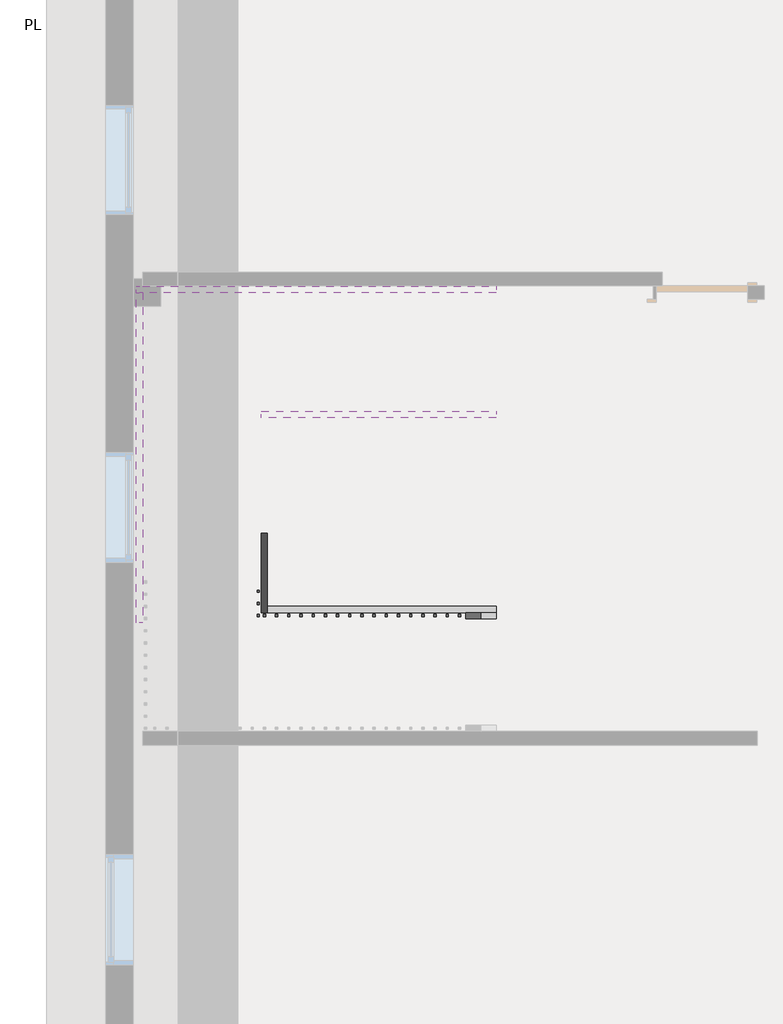
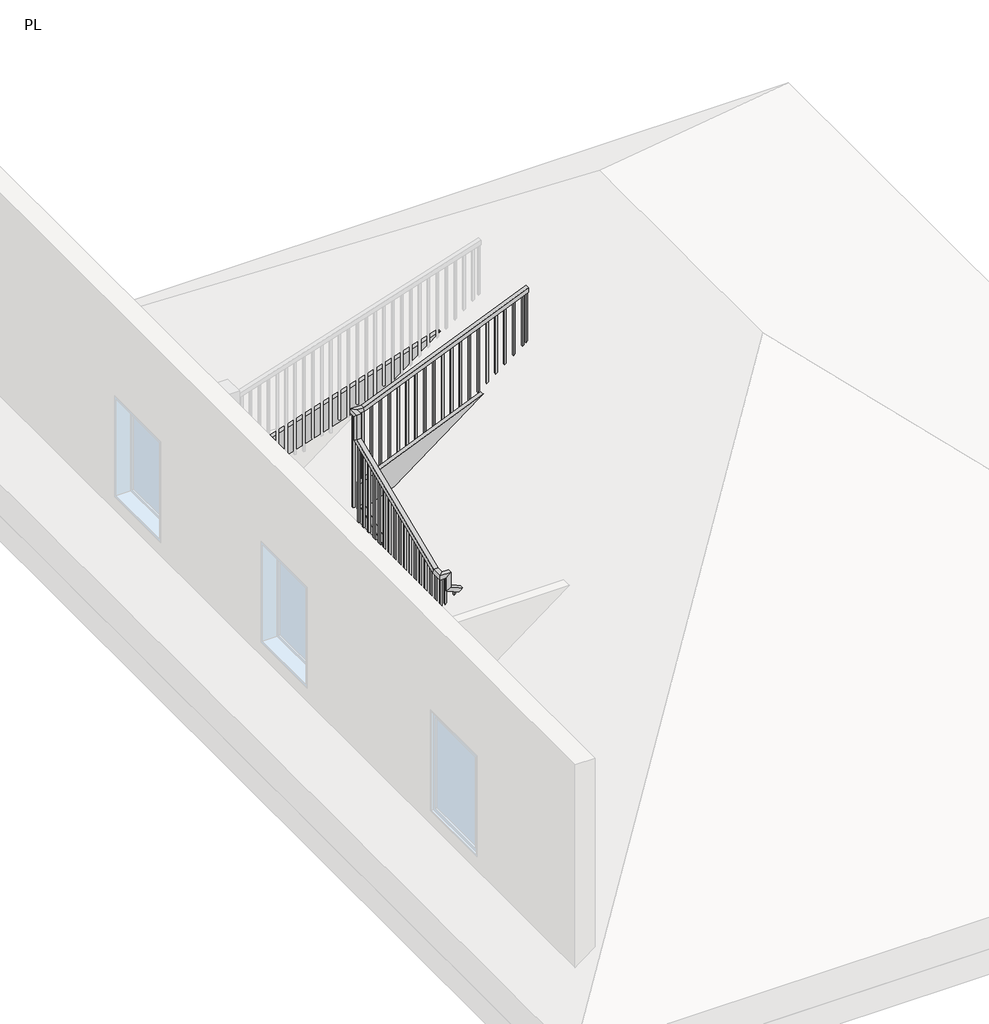
# One storey, part 3 of 3: 6 members, 1 railing.
"""IFC4 building model written with IfcOpenShell, lengths in millimetres."""

from ifc_helpers import new_model, si_unit, frame, origin, place, context, project, spatial, polyline, outline, extrude, faceted_brep, element, save

model = new_model("IFC4")

# Units and contexts
model_context = context("Model", 3, world=origin())
ifc_project = project(units=[si_unit("LENGTHUNIT", "METRE", prefix="MILLI")], contexts=[model_context])

# Site, building, storey
site = spatial("IfcSite", under=ifc_project)
building = spatial("IfcBuilding", under=site)
storey = spatial("IfcBuildingStorey", under=building, Name="PL", Elevation=0.0)

# Members
placement = place(None, origin())
element("IfcMember", 1, ObjectType="Stringer - 2\" Width", at=placement, inside=storey, context=model_context, shape_type="SweptSolid", body=[
    extrude(outline(polyline([(0.0, 5202.3334712), (314.7886477, 5202.3334712), (942.1719103, 3707.0700288), (942.1719103, 2919.2768366), (0.0, 5164.7865561), (0.0, 5202.3334712)])), frame((0.0, 4060.0450307, 0.0), z_axis=(0.0, 1.0, 0.0), x_axis=(0.0, 0.0, 1.0)), (0.0, 0.0, 1.0), 50.8),
])
element("IfcMember", 2, ObjectType="Stringer - 2\" Width", at=placement, inside=storey, context=model_context, shape_type="SweptSolid", body=[
    extrude(outline(polyline([(5015.4041654, 1220.4977979), (7768.4450307, 2067.5872949), (7768.4450307, 1748.6851248), (6051.8362182, 1220.4977979), (5015.4041654, 1220.4977979)])), frame((2205.1334712, 0.0, 0.0), z_axis=(1.0, 0.0, 0.0), x_axis=(0.0, 1.0, 0.0)), (0.0, 0.0, 1.0), 50.8),
])
element("IfcMember", 3, ObjectType="Stringer - 2\" Width", at=placement, inside=storey, context=model_context, shape_type="SweptSolid", body=[
    extrude(outline(polyline([(2051.8454089, 2205.1334712), (1748.6851248, 2205.1334712), (1748.6851248, 2257.6240611), (2685.9931599, 5202.3334712), (3005.8613241, 5202.3334712), (2051.8454089, 2205.1334712)])), frame((0.0, 7768.4450307, 0.0), z_axis=(0.0, 1.0, 0.0), x_axis=(0.0, 0.0, 1.0)), (0.0, 0.0, 1.0), 50.8),
])
element("IfcMember", 4, ObjectType="Stringer - 2\" Width", at=placement, inside=storey, context=model_context, shape_type="SweptSolid", body=[
    extrude(outline(polyline([(0.0, 5202.3334712), (314.7886477, 5202.3334712), (1114.089347, 3297.3334712), (783.5467489, 3297.3334712), (0.0, 5164.7865562), (0.0, 5202.3334712)])), frame((0.0, 5101.4450307, 0.0), z_axis=(0.0, 1.0, 0.0), x_axis=(0.0, 0.0, 1.0)), (0.0, 0.0, 1.0), 50.8),
])
element("IfcMember", 5, ObjectType="Stringer - 2\" Width", at=placement, inside=storey, context=model_context, shape_type="SweptSolid", body=[
    extrude(outline(polyline([(5101.4450307, 922.0922035), (5101.4450307, 1252.6348016), (6727.0450307, 1934.7047317), (6727.0450307, 1604.1621336), (5101.4450307, 922.0922035)])), frame((3246.5334712, 0.0, 0.0), z_axis=(1.0, 0.0, 0.0), x_axis=(0.0, 1.0, 0.0)), (0.0, 0.0, 1.0), 50.8),
])
element("IfcMember", 6, ObjectType="Stringer - 2\" Width", at=placement, inside=storey, context=model_context, shape_type="SweptSolid", body=[
    extrude(outline(polyline([(2190.4809554, 3246.5334712), (1859.9383573, 3246.5334712), (2680.5537419, 5202.3334712), (3011.0963401, 5202.3334712), (2190.4809554, 3246.5334712)])), frame((0.0, 6727.0450307, 0.0), z_axis=(0.0, 1.0, 0.0), x_axis=(0.0, 0.0, 1.0)), (0.0, 0.0, 1.0), 50.8),
])

# Railing
element("IfcRailing", 7, ObjectType="Handrail - Rectangular", at=placement, inside=storey, context=model_context, shape_type="SolidModel", body=[
    faceted_brep([(5202.3334712, 5050.6450307, 1148.8615385), (5202.3334712, 5050.6450307, 1093.7711054), (5202.3334712, 5101.4450307, 1093.7711054), (5202.3334712, 5101.4450307, 1148.8615385), (3322.7334712, 5050.6450307, 1937.5048951), (3271.9334712, 5050.6450307, 1903.7291474), (3271.9334712, 5101.4450307, 1903.7291474), (3322.7334712, 5101.4450307, 1937.5048951), (3322.7334712, 5050.6450307, 2118.6797203), (3271.9334712, 5050.6450307, 2067.8797203), (3271.9334712, 5101.4450307, 2067.8797203), (3322.7334712, 5101.4450307, 2118.6797203), (3195.7334712, 5050.6450307, 2118.6797203), (3195.7334712, 5050.6450307, 2067.8797203), (3246.5334712, 5101.4450307, 2067.8797203), (3246.5334712, 5101.4450307, 2118.6797203), (3195.7334712, 5177.6450307, 2118.6797203), (3195.7334712, 5187.8705627, 2067.8797203), (3246.5334712, 5187.8705627, 2067.8797203), (3246.5334712, 5177.6450307, 2118.6797203), (3195.7334712, 6701.6450307, 2758.1202797), (3195.7334712, 6752.4450307, 2724.344532), (3246.5334712, 6752.4450307, 2724.344532), (3246.5334712, 6701.6450307, 2758.1202797), (5202.3334712, 6828.6450307, 3845.1692308), (5202.3334712, 6777.8450307, 3845.1692308), (5202.3334712, 6777.8450307, 3790.0787978), (5202.3334712, 6828.6450307, 3790.0787978), (3332.9590032, 6828.6450307, 3005.7258741), (3322.7334712, 6828.6450307, 3056.5258741), (3332.9590032, 6777.8450307, 3005.7258741), (3322.7334712, 6777.8450307, 3056.5258741), (3195.7334712, 6701.6450307, 3056.5258741), (3195.7334712, 6752.4450307, 3005.7258741), (3246.5334712, 6752.4450307, 3005.7258741), (3246.5334712, 6701.6450307, 3056.5258741), (3195.7334712, 6828.6450307, 3056.5258741), (3195.7334712, 6828.6450307, 3005.7258741), (3246.5334712, 6777.8450307, 3005.7258741), (3246.5334712, 6777.8450307, 3056.5258741)], [[[0, 1, 2, 3]], [[1, 0, 4, 5]], [[2, 1, 5, 6]], [[3, 2, 6, 7]], [[0, 3, 7, 4]], [[5, 4, 8, 9]], [[6, 5, 9, 10]], [[7, 6, 10, 11]], [[4, 7, 11, 8]], [[9, 8, 12, 13]], [[10, 9, 13, 14]], [[11, 10, 14, 15]], [[8, 11, 15, 12]], [[13, 12, 16, 17]], [[14, 13, 17, 18]], [[15, 14, 18, 19]], [[12, 15, 19, 16]], [[17, 16, 20, 21]], [[18, 17, 21, 22]], [[19, 18, 22, 23]], [[16, 19, 23, 20]], [[24, 25, 26, 27]], [[28, 29, 24, 27]], [[30, 28, 27, 26]], [[31, 30, 26, 25]], [[29, 31, 25, 24]], [[21, 20, 32, 33]], [[22, 21, 33, 34]], [[23, 22, 34, 35]], [[20, 23, 35, 32]], [[33, 32, 36, 37]], [[34, 33, 37, 38]], [[35, 34, 38, 39]], [[32, 35, 39, 36]], [[37, 36, 29, 28]], [[38, 37, 28, 30]], [[39, 38, 30, 31]], [[36, 39, 31, 29]]]),
    extrude(outline(polyline([(3772.7606159, 5161.0584712), (3764.7676089, 5142.0084712), (2813.5384615, 5142.0084712), (2813.5384615, 5161.0584712), (3772.7606159, 5161.0584712)])), frame((0.0, 6793.7200307, 0.0), z_axis=(0.0, 1.0, 0.0), x_axis=(0.0, 0.0, 1.0)), (0.0, 0.0, 1.0), 19.05),
    extrude(outline(polyline([(3730.1312453, 5059.4584712), (3722.1382383, 5040.4084712), (2813.5384615, 5040.4084712), (2813.5384615, 5059.4584712), (3730.1312453, 5059.4584712)])), frame((0.0, 6793.7200307, 0.0), z_axis=(0.0, 1.0, 0.0), x_axis=(0.0, 0.0, 1.0)), (0.0, 0.0, 1.0), 19.05),
    extrude(outline(polyline([(3687.5018747, 4957.8584712), (3679.5088677, 4938.8084712), (2813.5384615, 4938.8084712), (2813.5384615, 4957.8584712), (3687.5018747, 4957.8584712)])), frame((0.0, 6793.7200307, 0.0), z_axis=(0.0, 1.0, 0.0), x_axis=(0.0, 0.0, 1.0)), (0.0, 0.0, 1.0), 19.05),
    extrude(outline(polyline([(3644.872504, 4856.2584712), (3636.8794971, 4837.2084712), (2696.3076923, 4837.2084712), (2696.3076923, 4856.2584712), (3644.872504, 4856.2584712)])), frame((0.0, 6793.7200307, 0.0), z_axis=(0.0, 1.0, 0.0), x_axis=(0.0, 0.0, 1.0)), (0.0, 0.0, 1.0), 19.05),
    extrude(outline(polyline([(3602.2431334, 4754.6584712), (3594.2501264, 4735.6084712), (2696.3076923, 4735.6084712), (2696.3076923, 4754.6584712), (3602.2431334, 4754.6584712)])), frame((0.0, 6793.7200307, 0.0), z_axis=(0.0, 1.0, 0.0), x_axis=(0.0, 0.0, 1.0)), (0.0, 0.0, 1.0), 19.05),
    extrude(outline(polyline([(3559.6137628, 4653.0584712), (3551.6207558, 4634.0084712), (2696.3076923, 4634.0084712), (2696.3076923, 4653.0584712), (3559.6137628, 4653.0584712)])), frame((0.0, 6793.7200307, 0.0), z_axis=(0.0, 1.0, 0.0), x_axis=(0.0, 0.0, 1.0)), (0.0, 0.0, 1.0), 19.05),
    extrude(outline(polyline([(3516.9843922, 4551.4584712), (3508.9913852, 4532.4084712), (2579.0769231, 4532.4084712), (2579.0769231, 4551.4584712), (3516.9843922, 4551.4584712)])), frame((0.0, 6793.7200307, 0.0), z_axis=(0.0, 1.0, 0.0), x_axis=(0.0, 0.0, 1.0)), (0.0, 0.0, 1.0), 19.05),
    extrude(outline(polyline([(3474.3550215, 4449.8584712), (3466.3620145, 4430.8084712), (2579.0769231, 4430.8084712), (2579.0769231, 4449.8584712), (3474.3550215, 4449.8584712)])), frame((0.0, 6793.7200307, 0.0), z_axis=(0.0, 1.0, 0.0), x_axis=(0.0, 0.0, 1.0)), (0.0, 0.0, 1.0), 19.05),
    extrude(outline(polyline([(3431.7256509, 4348.2584712), (3423.7326439, 4329.2084712), (2461.8461538, 4329.2084712), (2461.8461538, 4348.2584712), (3431.7256509, 4348.2584712)])), frame((0.0, 6793.7200307, 0.0), z_axis=(0.0, 1.0, 0.0), x_axis=(0.0, 0.0, 1.0)), (0.0, 0.0, 1.0), 19.05),
    extrude(outline(polyline([(3389.0962803, 4246.6584712), (3381.1032733, 4227.6084712), (2461.8461538, 4227.6084712), (2461.8461538, 4246.6584712), (3389.0962803, 4246.6584712)])), frame((0.0, 6793.7200307, 0.0), z_axis=(0.0, 1.0, 0.0), x_axis=(0.0, 0.0, 1.0)), (0.0, 0.0, 1.0), 19.05),
    extrude(outline(polyline([(3346.4669096, 4145.0584712), (3338.4739026, 4126.0084712), (2461.8461538, 4126.0084712), (2461.8461538, 4145.0584712), (3346.4669096, 4145.0584712)])), frame((0.0, 6793.7200307, 0.0), z_axis=(0.0, 1.0, 0.0), x_axis=(0.0, 0.0, 1.0)), (0.0, 0.0, 1.0), 19.05),
    extrude(outline(polyline([(3303.837539, 4043.4584712), (3295.844532, 4024.4084712), (2344.6153846, 4024.4084712), (2344.6153846, 4043.4584712), (3303.837539, 4043.4584712)])), frame((0.0, 6793.7200307, 0.0), z_axis=(0.0, 1.0, 0.0), x_axis=(0.0, 0.0, 1.0)), (0.0, 0.0, 1.0), 19.05),
    extrude(outline(polyline([(3261.2081684, 3941.8584712), (3253.2151614, 3922.8084712), (2344.6153846, 3922.8084712), (2344.6153846, 3941.8584712), (3261.2081684, 3941.8584712)])), frame((0.0, 6793.7200307, 0.0), z_axis=(0.0, 1.0, 0.0), x_axis=(0.0, 0.0, 1.0)), (0.0, 0.0, 1.0), 19.05),
    extrude(outline(polyline([(3218.5787978, 3840.2584712), (3210.5857908, 3821.2084712), (2344.6153846, 3821.2084712), (2344.6153846, 3840.2584712), (3218.5787978, 3840.2584712)])), frame((0.0, 6793.7200307, 0.0), z_axis=(0.0, 1.0, 0.0), x_axis=(0.0, 0.0, 1.0)), (0.0, 0.0, 1.0), 19.05),
    extrude(outline(polyline([(3175.9494271, 3738.6584712), (3167.9564201, 3719.6084712), (2227.3846154, 3719.6084712), (2227.3846154, 3738.6584712), (3175.9494271, 3738.6584712)])), frame((0.0, 6793.7200307, 0.0), z_axis=(0.0, 1.0, 0.0), x_axis=(0.0, 0.0, 1.0)), (0.0, 0.0, 1.0), 19.05),
    extrude(outline(polyline([(3133.3200565, 3637.0584712), (3125.3270495, 3618.0084712), (2227.3846154, 3618.0084712), (2227.3846154, 3637.0584712), (3133.3200565, 3637.0584712)])), frame((0.0, 6793.7200307, 0.0), z_axis=(0.0, 1.0, 0.0), x_axis=(0.0, 0.0, 1.0)), (0.0, 0.0, 1.0), 19.05),
    extrude(outline(polyline([(3090.6906859, 3535.4584712), (3082.6976789, 3516.4084712), (2227.3846154, 3516.4084712), (2227.3846154, 3535.4584712), (3090.6906859, 3535.4584712)])), frame((0.0, 6793.7200307, 0.0), z_axis=(0.0, 1.0, 0.0), x_axis=(0.0, 0.0, 1.0)), (0.0, 0.0, 1.0), 19.05),
    extrude(outline(polyline([(3048.0613152, 3433.8584712), (3040.0683082, 3414.8084712), (2110.1538462, 3414.8084712), (2110.1538462, 3433.8584712), (3048.0613152, 3433.8584712)])), frame((0.0, 6793.7200307, 0.0), z_axis=(0.0, 1.0, 0.0), x_axis=(0.0, 0.0, 1.0)), (0.0, 0.0, 1.0), 19.05),
    extrude(outline(polyline([(3005.4319446, 3332.2584712), (2997.4389376, 3313.2084712), (2110.1538462, 3313.2084712), (2110.1538462, 3332.2584712), (3005.4319446, 3332.2584712)])), frame((0.0, 6793.7200307, 0.0), z_axis=(0.0, 1.0, 0.0), x_axis=(0.0, 0.0, 1.0)), (0.0, 0.0, 1.0), 19.05),
    extrude(outline(polyline([(6692.1200307, 2699.0333432), (6711.1700307, 2707.0263502), (6711.1700307, 1758.4615385), (6692.1200307, 1758.4615385), (6692.1200307, 2699.0333432)])), frame((3211.6084712, 0.0, 0.0), z_axis=(1.0, 0.0, 0.0), x_axis=(0.0, 1.0, 0.0)), (0.0, 0.0, 1.0), 19.05),
    extrude(outline(polyline([(6590.5200307, 2656.4039726), (6609.5700307, 2664.3969796), (6609.5700307, 1758.4615385), (6590.5200307, 1758.4615385), (6590.5200307, 2656.4039726)])), frame((3211.6084712, 0.0, 0.0), z_axis=(1.0, 0.0, 0.0), x_axis=(0.0, 1.0, 0.0)), (0.0, 0.0, 1.0), 19.05),
    extrude(outline(polyline([(6488.9200307, 2613.7746019), (6507.9700307, 2621.7676089), (6507.9700307, 1758.4615385), (6488.9200307, 1758.4615385), (6488.9200307, 2613.7746019)])), frame((3211.6084712, 0.0, 0.0), z_axis=(1.0, 0.0, 0.0), x_axis=(0.0, 1.0, 0.0)), (0.0, 0.0, 1.0), 19.05),
    extrude(outline(polyline([(6387.3200307, 2571.1452313), (6406.3700307, 2579.1382383), (6406.3700307, 1641.2307692), (6387.3200307, 1641.2307692), (6387.3200307, 2571.1452313)])), frame((3211.6084712, 0.0, 0.0), z_axis=(1.0, 0.0, 0.0), x_axis=(0.0, 1.0, 0.0)), (0.0, 0.0, 1.0), 19.05),
    extrude(outline(polyline([(6285.7200307, 2528.5158607), (6304.7700307, 2536.5088677), (6304.7700307, 1641.2307692), (6285.7200307, 1641.2307692), (6285.7200307, 2528.5158607)])), frame((3211.6084712, 0.0, 0.0), z_axis=(1.0, 0.0, 0.0), x_axis=(0.0, 1.0, 0.0)), (0.0, 0.0, 1.0), 19.05),
    extrude(outline(polyline([(6184.1200307, 2485.8864901), (6203.1700307, 2493.8794971), (6203.1700307, 1524.0), (6184.1200307, 1524.0), (6184.1200307, 2485.8864901)])), frame((3211.6084712, 0.0, 0.0), z_axis=(1.0, 0.0, 0.0), x_axis=(0.0, 1.0, 0.0)), (0.0, 0.0, 1.0), 19.05),
    extrude(outline(polyline([(6082.5200307, 2443.2571194), (6101.5700307, 2451.2501264), (6101.5700307, 1524.0), (6082.5200307, 1524.0), (6082.5200307, 2443.2571194)])), frame((3211.6084712, 0.0, 0.0), z_axis=(1.0, 0.0, 0.0), x_axis=(0.0, 1.0, 0.0)), (0.0, 0.0, 1.0), 19.05),
    extrude(outline(polyline([(5980.9200307, 2400.6277488), (5999.9700307, 2408.6207558), (5999.9700307, 1524.0), (5980.9200307, 1524.0), (5980.9200307, 2400.6277488)])), frame((3211.6084712, 0.0, 0.0), z_axis=(1.0, 0.0, 0.0), x_axis=(0.0, 1.0, 0.0)), (0.0, 0.0, 1.0), 19.05),
    extrude(outline(polyline([(5879.3200307, 2357.9983782), (5898.3700307, 2365.9913852), (5898.3700307, 1406.7692308), (5879.3200307, 1406.7692308), (5879.3200307, 2357.9983782)])), frame((3211.6084712, 0.0, 0.0), z_axis=(1.0, 0.0, 0.0), x_axis=(0.0, 1.0, 0.0)), (0.0, 0.0, 1.0), 19.05),
    extrude(outline(polyline([(5777.7200307, 2315.3690075), (5796.7700307, 2323.3620145), (5796.7700307, 1406.7692308), (5777.7200307, 1406.7692308), (5777.7200307, 2315.3690075)])), frame((3211.6084712, 0.0, 0.0), z_axis=(1.0, 0.0, 0.0), x_axis=(0.0, 1.0, 0.0)), (0.0, 0.0, 1.0), 19.05),
    extrude(outline(polyline([(5676.1200307, 2272.7396369), (5695.1700307, 2280.7326439), (5695.1700307, 1406.7692308), (5676.1200307, 1406.7692308), (5676.1200307, 2272.7396369)])), frame((3211.6084712, 0.0, 0.0), z_axis=(1.0, 0.0, 0.0), x_axis=(0.0, 1.0, 0.0)), (0.0, 0.0, 1.0), 19.05),
    extrude(outline(polyline([(5574.5200307, 2230.1102663), (5593.5700307, 2238.1032733), (5593.5700307, 1289.5384615), (5574.5200307, 1289.5384615), (5574.5200307, 2230.1102663)])), frame((3211.6084712, 0.0, 0.0), z_axis=(1.0, 0.0, 0.0), x_axis=(0.0, 1.0, 0.0)), (0.0, 0.0, 1.0), 19.05),
    extrude(outline(polyline([(5472.9200307, 2187.4808957), (5491.9700307, 2195.4739026), (5491.9700307, 1289.5384615), (5472.9200307, 1289.5384615), (5472.9200307, 2187.4808957)])), frame((3211.6084712, 0.0, 0.0), z_axis=(1.0, 0.0, 0.0), x_axis=(0.0, 1.0, 0.0)), (0.0, 0.0, 1.0), 19.05),
    extrude(outline(polyline([(5371.3200307, 2144.851525), (5390.3700307, 2152.844532), (5390.3700307, 1289.5384615), (5371.3200307, 1289.5384615), (5371.3200307, 2144.851525)])), frame((3211.6084712, 0.0, 0.0), z_axis=(1.0, 0.0, 0.0), x_axis=(0.0, 1.0, 0.0)), (0.0, 0.0, 1.0), 19.05),
    extrude(outline(polyline([(5269.7200307, 2102.2221544), (5288.7700307, 2110.2151614), (5288.7700307, 1172.3076923), (5269.7200307, 1172.3076923), (5269.7200307, 2102.2221544)])), frame((3211.6084712, 0.0, 0.0), z_axis=(1.0, 0.0, 0.0), x_axis=(0.0, 1.0, 0.0)), (0.0, 0.0, 1.0), 19.05),
    extrude(outline(polyline([(5168.1200307, 2059.5927838), (5187.1700307, 2067.5857908), (5187.1700307, 1172.3076923), (5168.1200307, 1172.3076923), (5168.1200307, 2059.5927838)])), frame((3211.6084712, 0.0, 0.0), z_axis=(1.0, 0.0, 0.0), x_axis=(0.0, 1.0, 0.0)), (0.0, 0.0, 1.0), 19.05),
    extrude(outline(polyline([(3281.4584712, 5085.5700307), (3281.4584712, 5066.5200307), (3262.4084712, 5066.5200307), (3262.4084712, 5085.5700307), (3281.4584712, 5085.5700307)])), frame((0.0, 0.0, 937.8461538), z_axis=(0.0, 0.0, 1.0), x_axis=(1.0, 0.0, 0.0)), (0.0, 0.0, 1.0), 1130.0335664),
    extrude(outline(polyline([(1857.1032733, 3383.0584712), (1865.0962803, 3364.0084712), (937.8461538, 3364.0084712), (937.8461538, 3383.0584712), (1857.1032733, 3383.0584712)])), frame((0.0, 5066.5200307, 0.0), z_axis=(0.0, 1.0, 0.0), x_axis=(0.0, 0.0, 1.0)), (0.0, 0.0, 1.0), 19.05),
    extrude(outline(polyline([(1814.4739026, 3484.6584712), (1822.4669096, 3465.6084712), (937.8461538, 3465.6084712), (937.8461538, 3484.6584712), (1814.4739026, 3484.6584712)])), frame((0.0, 5066.5200307, 0.0), z_axis=(0.0, 1.0, 0.0), x_axis=(0.0, 0.0, 1.0)), (0.0, 0.0, 1.0), 19.05),
    extrude(outline(polyline([(1771.844532, 3586.2584712), (1779.837539, 3567.2084712), (820.6153846, 3567.2084712), (820.6153846, 3586.2584712), (1771.844532, 3586.2584712)])), frame((0.0, 5066.5200307, 0.0), z_axis=(0.0, 1.0, 0.0), x_axis=(0.0, 0.0, 1.0)), (0.0, 0.0, 1.0), 19.05),
    extrude(outline(polyline([(1729.2151614, 3687.8584712), (1737.2081684, 3668.8084712), (820.6153846, 3668.8084712), (820.6153846, 3687.8584712), (1729.2151614, 3687.8584712)])), frame((0.0, 5066.5200307, 0.0), z_axis=(0.0, 1.0, 0.0), x_axis=(0.0, 0.0, 1.0)), (0.0, 0.0, 1.0), 19.05),
    extrude(outline(polyline([(1686.5857908, 3789.4584712), (1694.5787978, 3770.4084712), (820.6153846, 3770.4084712), (820.6153846, 3789.4584712), (1686.5857908, 3789.4584712)])), frame((0.0, 5066.5200307, 0.0), z_axis=(0.0, 1.0, 0.0), x_axis=(0.0, 0.0, 1.0)), (0.0, 0.0, 1.0), 19.05),
    extrude(outline(polyline([(1643.9564201, 3891.0584712), (1651.9494271, 3872.0084712), (703.3846154, 3872.0084712), (703.3846154, 3891.0584712), (1643.9564201, 3891.0584712)])), frame((0.0, 5066.5200307, 0.0), z_axis=(0.0, 1.0, 0.0), x_axis=(0.0, 0.0, 1.0)), (0.0, 0.0, 1.0), 19.05),
    extrude(outline(polyline([(1601.3270495, 3992.6584712), (1609.3200565, 3973.6084712), (703.3846154, 3973.6084712), (703.3846154, 3992.6584712), (1601.3270495, 3992.6584712)])), frame((0.0, 5066.5200307, 0.0), z_axis=(0.0, 1.0, 0.0), x_axis=(0.0, 0.0, 1.0)), (0.0, 0.0, 1.0), 19.05),
    extrude(outline(polyline([(1558.6976789, 4094.2584712), (1566.6906859, 4075.2084712), (703.3846154, 4075.2084712), (703.3846154, 4094.2584712), (1558.6976789, 4094.2584712)])), frame((0.0, 5066.5200307, 0.0), z_axis=(0.0, 1.0, 0.0), x_axis=(0.0, 0.0, 1.0)), (0.0, 0.0, 1.0), 19.05),
    extrude(outline(polyline([(1516.0683082, 4195.8584712), (1524.0613152, 4176.8084712), (586.1538462, 4176.8084712), (586.1538462, 4195.8584712), (1516.0683082, 4195.8584712)])), frame((0.0, 5066.5200307, 0.0), z_axis=(0.0, 1.0, 0.0), x_axis=(0.0, 0.0, 1.0)), (0.0, 0.0, 1.0), 19.05),
    extrude(outline(polyline([(1473.4389376, 4297.4584712), (1481.4319446, 4278.4084712), (586.1538462, 4278.4084712), (586.1538462, 4297.4584712), (1473.4389376, 4297.4584712)])), frame((0.0, 5066.5200307, 0.0), z_axis=(0.0, 1.0, 0.0), x_axis=(0.0, 0.0, 1.0)), (0.0, 0.0, 1.0), 19.05),
    extrude(outline(polyline([(1430.809567, 4399.0584712), (1438.802574, 4380.0084712), (468.9230769, 4380.0084712), (468.9230769, 4399.0584712), (1430.809567, 4399.0584712)])), frame((0.0, 5066.5200307, 0.0), z_axis=(0.0, 1.0, 0.0), x_axis=(0.0, 0.0, 1.0)), (0.0, 0.0, 1.0), 19.05),
    extrude(outline(polyline([(1388.1801964, 4500.6584712), (1396.1732033, 4481.6084712), (468.9230769, 4481.6084712), (468.9230769, 4500.6584712), (1388.1801964, 4500.6584712)])), frame((0.0, 5066.5200307, 0.0), z_axis=(0.0, 1.0, 0.0), x_axis=(0.0, 0.0, 1.0)), (0.0, 0.0, 1.0), 19.05),
    extrude(outline(polyline([(1345.5508257, 4602.2584712), (1353.5438327, 4583.2084712), (468.9230769, 4583.2084712), (468.9230769, 4602.2584712), (1345.5508257, 4602.2584712)])), frame((0.0, 5066.5200307, 0.0), z_axis=(0.0, 1.0, 0.0), x_axis=(0.0, 0.0, 1.0)), (0.0, 0.0, 1.0), 19.05),
    extrude(outline(polyline([(1302.9214551, 4703.8584712), (1310.9144621, 4684.8084712), (351.6923077, 4684.8084712), (351.6923077, 4703.8584712), (1302.9214551, 4703.8584712)])), frame((0.0, 5066.5200307, 0.0), z_axis=(0.0, 1.0, 0.0), x_axis=(0.0, 0.0, 1.0)), (0.0, 0.0, 1.0), 19.05),
    extrude(outline(polyline([(1260.2920845, 4805.4584712), (1268.2850915, 4786.4084712), (351.6923077, 4786.4084712), (351.6923077, 4805.4584712), (1260.2920845, 4805.4584712)])), frame((0.0, 5066.5200307, 0.0), z_axis=(0.0, 1.0, 0.0), x_axis=(0.0, 0.0, 1.0)), (0.0, 0.0, 1.0), 19.05),
    extrude(outline(polyline([(1217.6627138, 4907.0584712), (1225.6557208, 4888.0084712), (351.6923077, 4888.0084712), (351.6923077, 4907.0584712), (1217.6627138, 4907.0584712)])), frame((0.0, 5066.5200307, 0.0), z_axis=(0.0, 1.0, 0.0), x_axis=(0.0, 0.0, 1.0)), (0.0, 0.0, 1.0), 19.05),
    extrude(outline(polyline([(1175.0333432, 5008.6584712), (1183.0263502, 4989.6084712), (234.4615385, 4989.6084712), (234.4615385, 5008.6584712), (1175.0333432, 5008.6584712)])), frame((0.0, 5066.5200307, 0.0), z_axis=(0.0, 1.0, 0.0), x_axis=(0.0, 0.0, 1.0)), (0.0, 0.0, 1.0), 19.05),
    extrude(outline(polyline([(1132.4039726, 5110.2584712), (1140.3969796, 5091.2084712), (234.4615385, 5091.2084712), (234.4615385, 5110.2584712), (1132.4039726, 5110.2584712)])), frame((0.0, 5066.5200307, 0.0), z_axis=(0.0, 1.0, 0.0), x_axis=(0.0, 0.0, 1.0)), (0.0, 0.0, 1.0), 19.05),
    extrude(outline(polyline([(3230.6584712, 6793.7200307), (3211.6084712, 6793.7200307), (3211.6084712, 6812.7700307), (3230.6584712, 6812.7700307), (3230.6584712, 6793.7200307)])), frame((0.0, 0.0, 1875.6923077), z_axis=(0.0, 0.0, 1.0), x_axis=(1.0, 0.0, 0.0)), (0.0, 0.0, 1.0), 1130.0335664),
    extrude(outline(polyline([(3230.6584712, 5085.5700307), (3230.6584712, 5066.5200307), (3211.6084712, 5066.5200307), (3211.6084712, 5085.5700307), (3230.6584712, 5085.5700307)])), frame((0.0, 0.0, 1055.0769231), z_axis=(0.0, 0.0, 1.0), x_axis=(1.0, 0.0, 0.0)), (0.0, 0.0, 1.0), 1012.8027972),
    extrude(outline(polyline([(3790.0787978, 5202.3334712), (3782.0857908, 5183.2834712), (2930.7692308, 5183.2834712), (2930.7692308, 5202.3334712), (3790.0787978, 5202.3334712)])), frame((0.0, 6793.7200307, 0.0), z_axis=(0.0, 1.0, 0.0), x_axis=(0.0, 0.0, 1.0)), (0.0, 0.0, 1.0), 19.05),
    extrude(outline(polyline([(1093.7711054, 5202.3334712), (1101.7641124, 5183.2834712), (117.2307692, 5183.2834712), (117.2307692, 5202.3334712), (1093.7711054, 5202.3334712)])), frame((0.0, 5066.5200307, 0.0), z_axis=(0.0, 1.0, 0.0), x_axis=(0.0, 0.0, 1.0)), (0.0, 0.0, 1.0), 19.05),
])

save(model, "model.ifc")

# Revit data of these elements
# Type "Handrail - Rectangular"
#   Assembly Code = "C2010400"
#   built-in parameter 1008612 = 0.0416667 (stored number, unit not read)
#   built-in parameter 1008611 = 0.0416667 (stored number, unit not read)
#   built-in parameter 1008609 = 0.333333 (stored number, unit not read)
#   built-in parameter 1008604 = 0.166667 (stored number, unit not read)
#   built-in parameter 1008603 = 0.166667 (stored number, unit not read)
#   Railing Height = 3' - 0"
#   built-in parameter 1008630 = 2
#   built-in parameter 1008610 = 2
#   built-in parameter 1008618 = Baluster - Square : 3/4"
# Elements 1, 2, 3, 4, 5, 6 (IfcMember, "Stringer - 2\" Width")
#   Phase Created = New Construction
# Element 7 (IfcRailing, "Handrail - Rectangular")
#   Phase Created = New Construction
